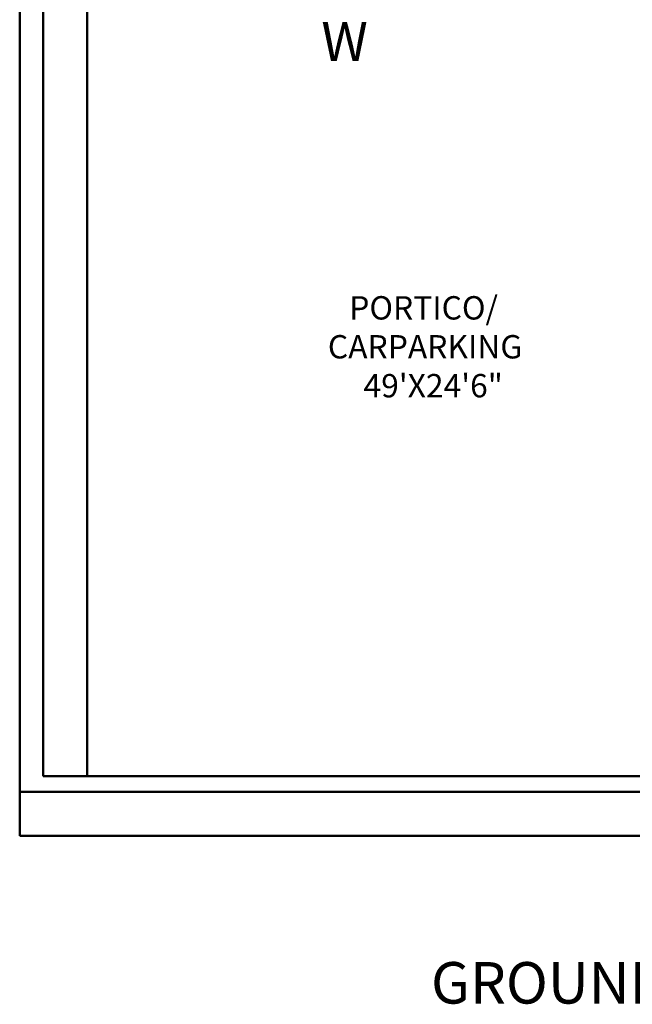
# Model space of a CAD drawing. Units: inches. Extents: x -7040 to -4088, y 6092 to 7645.
# Tile 1 of 11: x -7003 to -6767, y 6092 to 6471. Entities that reach past the tile are written whole.
import ezdxf

# ---------------------------------------------------------------- set-up
doc = ezdxf.new("R2010")
doc.units = ezdxf.units.IN
for name, color, linetype, lineweight in [('A-ANNO-TEXT', 7, 'Continuous', 25), ('A-AREA-IDEN', 3, 'Continuous', 25), ('A-WALL', 7, 'Continuous', 50)]:
    doc.layers.add(name, color=color, linetype=linetype, lineweight=lineweight)
doc.styles.get("Standard").update_dxf_attribs({"font": 'arial.ttf'})

msp = doc.modelspace()

# ---------------------------------------------------------------- linework, layer by layer
at = {"layer": 'A-WALL'}
for p, q in [((-7003.03, 6156.76), (-7003.03, 7513.76)), ((-6994.03, 6179.76), (-6994.03, 7504.76)), ((-6977.03, 6179.76), (-6977.03, 7487.76)), ((-6994.03, 6179.76), (-6412.03, 6179.76)), ((-7003.03, 6173.76), (-6403.03, 6173.76)), ((-7003.03, 6156.76), (-6403.03, 6156.76))]:
    msp.add_line(p, q, dxfattribs=at)

# ---------------------------------------------------------------- texts
at = {"layer": 'A-ANNO-TEXT', "attachment_point": 1}
for s, width, insert, char_height in [('{W}', 701.5203, (-6886.65, 6470.43), 15), ('{GROUND FLOOR PLAN}', 679.9892, (-6844.34, 6108.11), 16)]:
    msp.add_mtext_dynamic_manual_height_columns(s, width=width, gutter_width=12.5, heights=[0], dxfattribs=dict(at, insert=insert, char_height=char_height))
at = {"layer": 'A-AREA-IDEN', "insert": (-6884.13, 6364.75), "char_height": 9, "attachment_point": 1}
msp.add_mtext_dynamic_manual_height_columns('{   PORTICO/\\PCARPARKING\\P     49\'X24\'6"}', width=930.9751, gutter_width=12.5, heights=[0], dxfattribs=at)

doc.saveas('drawing.dxf')
